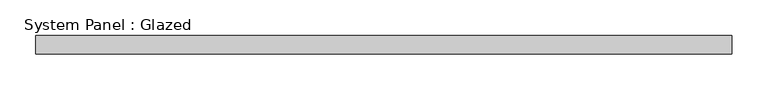
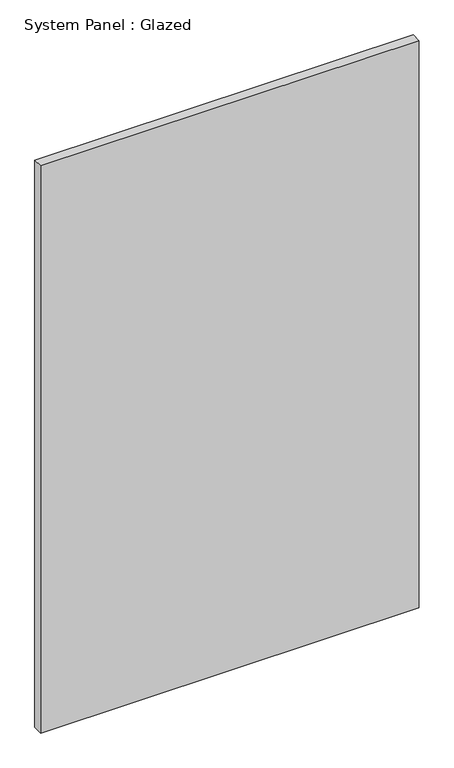
"""IFC4 building model written with IfcOpenShell, lengths in millimetres: plate geometry, System Panel : Glazed."""

from ifc_helpers import new_model, si_unit, origin, origin_with_axes, place, context, project, spatial, polyline, outline, extrude, source, transform, mapped, element, save


def system_panel_glazed_9cc53619(model_context):
    return source(origin(), model_context, "Body", "SweptSolid", [
        extrude(outline(polyline([(485.775, 19.05), (-485.775, 19.05), (-485.775, 44.45), (485.775, 44.45), (485.775, 19.05)])), origin_with_axes(), (0.0, 0.0, 1.0), 1538.3902237),
    ])


if __name__ == "__main__":
    model = new_model("IFC4")
    model_context = context("Model", 3, world=origin())
    ifc_project = project(units=[si_unit("LENGTHUNIT", "METRE", prefix="MILLI")], contexts=[model_context])
    site = spatial("IfcSite", under=ifc_project)
    building = spatial("IfcBuilding", under=site)
    placement = place(None, origin())
    system_panel_glazed_shape = system_panel_glazed_9cc53619(model_context)
    element("IfcPlate", 1, ObjectType="System Panel : Glazed", at=placement, inside=building, context=model_context, shape_type="MappedRepresentation", body=[
        mapped(system_panel_glazed_shape, transform((0.0, 0.0, 0.0), x_axis=(1.0, 0.0, 0.0), y_axis=(0.0, 1.0, 0.0), z_axis=(0.0, 0.0, 1.0))),
    ])
    save(model, "model.ifc")

# Revit data of these elements
# Type "System Panel : Glazed"
#   Construction Type Id = "GSP4R"
#   Analytic Construction = "1/8 in Pilkington single glazing"
#   Visual Light Transmittance = 0.9
#   Solar Heat Gain Coefficient = 0.86
#   Heat Transfer Coefficient (U) = 1.18115 BTU/(h·ft²·°F)
#   Define Thermal Properties by = 1
# Element 1 (IfcPlate, "System Panel : Glazed")
#   Materials on its faces: "Glass"
# Materials
#   "Glass": class "Glass", colour RGB 0 128 192, transparency 0.75, Description = "Soda Lime Glass", Cost = 0
